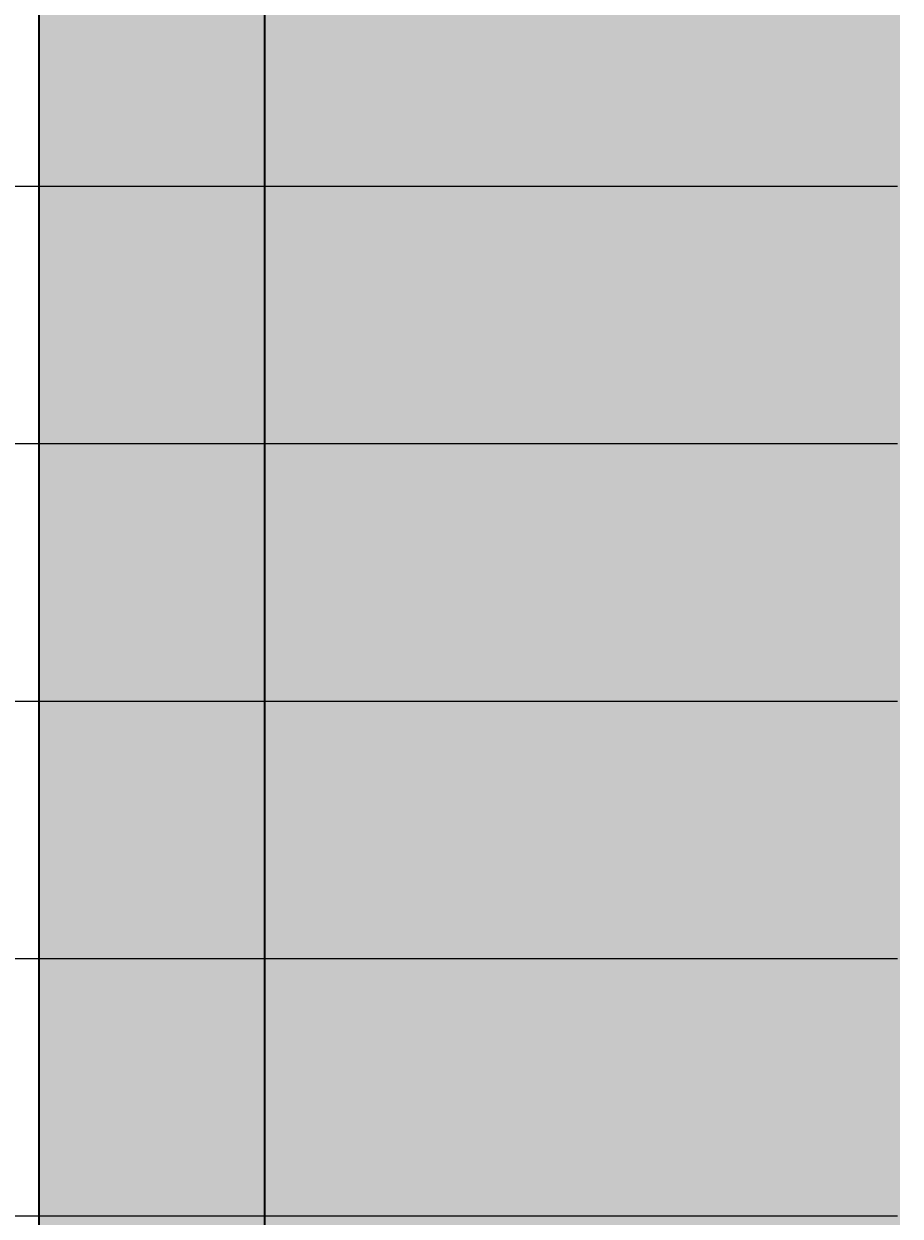
# Model space of a CAD drawing. Units: feet. Extents: x 2695 to 2912, y 795 to 1139.
# Tile 41 of 83: x 2710 to 2731, y 993 to 1020. Entities that reach past the tile are written whole.
import ezdxf

# ---------------------------------------------------------------- set-up
doc = ezdxf.new("R2010")
doc.units = ezdxf.units.FT
for name, color, linetype, lineweight in [('A-ANNO-DIMS', 2, 'Continuous', 18), ('A-ELEV', 7, 'Continuous', 35), ('A-ELEV-PATT', 252, 'Continuous', 13)]:
    doc.layers.add(name, color=color, linetype=linetype, lineweight=lineweight)
doc.styles.get("Standard").update_dxf_attribs({"font": 'arial.ttf'})
doc.dimstyles.get("Standard").update_dxf_attribs({"dimtxt": 0.18, "dimasz": 0.18, "dimexe": 0.18, "dimexo": 0.0625, "dimgap": 0.09, "dimtad": 0, "dimtih": 1, "dimtoh": 1, "dimdec": 1, "dimzin": 0, "dimdsep": 46, "dimlunit": 3, "dimtxsty": 'Standard', "dimcen": 0.09, "dimadec": 0, "dimazin": 0, "dimtfac": 1, "dimtdec": 1, "dimtofl": 0, "dimtmove": 0, "dimatfit": 3, "dimfxl": 1, "dimtolj": 1, "dimtzin": 0, "dimarcsym": 0})

# ---------------------------------------------------------------- blocks, each defined once
blk = doc.blocks.new('*D12')
at = {"layer": 'A-ANNO-DIMS', "color": 0, "lineweight": -2, "transparency": 16777216}
for p, q in [((2710.574, 1122.931), (2694.681, 1122.931)), ((2694.861, 1122.751), (2694.861, 967.113)), ((2694.861, 811.111), (2694.861, 966.749)), ((2710.574, 810.931), (2694.681, 810.931))]:
    blk.add_line(p, q, dxfattribs=at)
at = {"layer": 'A-ANNO-DIMS', "color": 0, "transparency": 16777216}
for points in [[(2694.831, 1122.751), (2694.891, 1122.751), (2694.861, 1122.931)], [(2694.831, 811.111), (2694.891, 811.111), (2694.861, 810.931)]]:
    blk.add_solid(points, dxfattribs=at)
at = {"layer": 'Defpoints', "color": 0, "transparency": 16777216}
for p in [(2694.861, 1122.931), (2710.636, 1122.931), (2710.636, 810.931)]:
    blk.add_point(p, dxfattribs=at)
at = {"layer": 'A-ANNO-DIMS', "color": 0, "transparency": 16777216, "insert": (2694.861, 966.931), "char_height": 0.18, "attachment_point": 5}
blk.add_mtext('\\A1;312', dxfattribs=at)
blk = doc.blocks.new('*D36')
at = {"layer": 'A-ANNO-DIMS', "color": 0, "lineweight": -2, "transparency": 16777216}
for p, q in [((2730.646, 992.518), (2694.681, 992.518)), ((2694.861, 992.338), (2694.861, 989.7)), ((2694.861, 986.698), (2694.861, 989.336)), ((2730.646, 986.518), (2694.681, 986.518))]:
    blk.add_line(p, q, dxfattribs=at)
at = {"layer": 'A-ANNO-DIMS', "color": 0, "transparency": 16777216}
for points in [[(2694.831, 992.338), (2694.891, 992.338), (2694.861, 992.518)], [(2694.831, 986.698), (2694.891, 986.698), (2694.861, 986.518)]]:
    blk.add_solid(points, dxfattribs=at)
at = {"layer": 'Defpoints', "color": 0, "transparency": 16777216}
for p in [(2694.861, 992.518), (2730.708, 992.518), (2730.708, 986.518)]:
    blk.add_point(p, dxfattribs=at)
at = {"layer": 'A-ANNO-DIMS', "color": 0, "transparency": 16777216, "insert": (2694.861, 989.518), "char_height": 0.18, "attachment_point": 5}
blk.add_mtext('\\A1;6', dxfattribs=at)
blk = doc.blocks.new('*D37')
at = {"layer": 'A-ANNO-DIMS', "color": 0, "lineweight": -2, "transparency": 16777216}
for p, q in [((2730.646, 998.518), (2694.681, 998.518)), ((2694.861, 998.338), (2694.861, 995.7)), ((2694.861, 992.698), (2694.861, 995.336)), ((2730.646, 992.518), (2694.681, 992.518))]:
    blk.add_line(p, q, dxfattribs=at)
at = {"layer": 'A-ANNO-DIMS', "color": 0, "transparency": 16777216}
for points in [[(2694.831, 998.338), (2694.891, 998.338), (2694.861, 998.518)], [(2694.831, 992.698), (2694.891, 992.698), (2694.861, 992.518)]]:
    blk.add_solid(points, dxfattribs=at)
at = {"layer": 'Defpoints', "color": 0, "transparency": 16777216}
for p in [(2694.861, 998.518), (2730.708, 998.518), (2730.708, 992.518)]:
    blk.add_point(p, dxfattribs=at)
at = {"layer": 'A-ANNO-DIMS', "color": 0, "transparency": 16777216, "insert": (2694.861, 995.518), "char_height": 0.18, "attachment_point": 5}
blk.add_mtext('\\A1;6', dxfattribs=at)
blk = doc.blocks.new('*D38')
at = {"layer": 'A-ANNO-DIMS', "color": 0, "lineweight": -2, "transparency": 16777216}
for p, q in [((2730.646, 1004.518), (2694.681, 1004.518)), ((2694.861, 1004.338), (2694.861, 1001.7)), ((2694.861, 998.698), (2694.861, 1001.336)), ((2730.646, 998.518), (2694.681, 998.518))]:
    blk.add_line(p, q, dxfattribs=at)
at = {"layer": 'A-ANNO-DIMS', "color": 0, "transparency": 16777216}
for points in [[(2694.831, 1004.338), (2694.891, 1004.338), (2694.861, 1004.518)], [(2694.831, 998.698), (2694.891, 998.698), (2694.861, 998.518)]]:
    blk.add_solid(points, dxfattribs=at)
at = {"layer": 'Defpoints', "color": 0, "transparency": 16777216}
for p in [(2694.861, 1004.518), (2730.708, 1004.518), (2730.708, 998.518)]:
    blk.add_point(p, dxfattribs=at)
at = {"layer": 'A-ANNO-DIMS', "color": 0, "transparency": 16777216, "insert": (2694.861, 1001.518), "char_height": 0.18, "attachment_point": 5}
blk.add_mtext('\\A1;6', dxfattribs=at)
blk = doc.blocks.new('*D39')
at = {"layer": 'A-ANNO-DIMS', "color": 0, "lineweight": -2, "transparency": 16777216}
for p, q in [((2730.646, 1010.518), (2694.681, 1010.518)), ((2694.861, 1010.338), (2694.861, 1007.7)), ((2694.861, 1004.698), (2694.861, 1007.336)), ((2730.646, 1004.518), (2694.681, 1004.518))]:
    blk.add_line(p, q, dxfattribs=at)
at = {"layer": 'A-ANNO-DIMS', "color": 0, "transparency": 16777216}
for points in [[(2694.831, 1010.338), (2694.891, 1010.338), (2694.861, 1010.518)], [(2694.831, 1004.698), (2694.891, 1004.698), (2694.861, 1004.518)]]:
    blk.add_solid(points, dxfattribs=at)
at = {"layer": 'Defpoints', "color": 0, "transparency": 16777216}
for p in [(2694.861, 1010.518), (2730.708, 1010.518), (2730.708, 1004.518)]:
    blk.add_point(p, dxfattribs=at)
at = {"layer": 'A-ANNO-DIMS', "color": 0, "transparency": 16777216, "insert": (2694.861, 1007.518), "char_height": 0.18, "attachment_point": 5}
blk.add_mtext('\\A1;6', dxfattribs=at)
blk = doc.blocks.new('*D40')
at = {"layer": 'A-ANNO-DIMS', "color": 0, "lineweight": -2, "transparency": 16777216}
for p, q in [((2730.646, 1016.518), (2694.681, 1016.518)), ((2694.861, 1016.338), (2694.861, 1013.7)), ((2694.861, 1010.698), (2694.861, 1013.336)), ((2730.646, 1010.518), (2694.681, 1010.518))]:
    blk.add_line(p, q, dxfattribs=at)
at = {"layer": 'A-ANNO-DIMS', "color": 0, "transparency": 16777216}
for points in [[(2694.831, 1016.338), (2694.891, 1016.338), (2694.861, 1016.518)], [(2694.831, 1010.698), (2694.891, 1010.698), (2694.861, 1010.518)]]:
    blk.add_solid(points, dxfattribs=at)
at = {"layer": 'Defpoints', "color": 0, "transparency": 16777216}
for p in [(2694.861, 1016.518), (2730.708, 1016.518), (2730.708, 1010.518)]:
    blk.add_point(p, dxfattribs=at)
at = {"layer": 'A-ANNO-DIMS', "color": 0, "transparency": 16777216, "insert": (2694.861, 1013.518), "char_height": 0.18, "attachment_point": 5}
blk.add_mtext('\\A1;6', dxfattribs=at)
blk = doc.blocks.new('*D41')
at = {"layer": 'A-ANNO-DIMS', "color": 0, "lineweight": -2, "transparency": 16777216}
for p, q in [((2730.646, 1022.518), (2694.681, 1022.518)), ((2694.861, 1022.338), (2694.861, 1019.7)), ((2694.861, 1016.698), (2694.861, 1019.336)), ((2730.646, 1016.518), (2694.681, 1016.518))]:
    blk.add_line(p, q, dxfattribs=at)
at = {"layer": 'A-ANNO-DIMS', "color": 0, "transparency": 16777216}
for points in [[(2694.831, 1022.338), (2694.891, 1022.338), (2694.861, 1022.518)], [(2694.831, 1016.698), (2694.891, 1016.698), (2694.861, 1016.518)]]:
    blk.add_solid(points, dxfattribs=at)
at = {"layer": 'Defpoints', "color": 0, "transparency": 16777216}
for p in [(2694.861, 1022.518), (2730.708, 1022.518), (2730.708, 1016.518)]:
    blk.add_point(p, dxfattribs=at)
at = {"layer": 'A-ANNO-DIMS', "color": 0, "transparency": 16777216, "insert": (2694.861, 1019.518), "char_height": 0.18, "attachment_point": 5}
blk.add_mtext('\\A1;6', dxfattribs=at)

msp = doc.modelspace()

# ---------------------------------------------------------------- hatches: boundary and pattern name
at = {"layer": 'A-ELEV-PATT'}
h = msp.add_hatch(color=256, dxfattribs=at)
h.set_gradient(color1=(255, 255, 255), tint=1)
h.paths.add_polyline_path([(2770.6361, 1122.9306), (2710.6361, 1122.9306), (2710.6361, 1118.4096), (2770.6361, 1118.4096)])
h.paths.add_polyline_path([(2890.6361, 1107.8588), (2770.6361, 1107.8588), (2770.6361, 1103.3378), (2890.6361, 1103.3378)])
h.paths.add_polyline_path([(2890.6361, 1062.9306), (2710.6361, 1062.9306), (2710.6361, 1056.9306), (2710.6361, 936.9306), (2710.6361, 924.3105), (2716.5358, 924.3105), (2890.6361, 924.3105), (2890.6361, 936.9306), (2715.8852, 936.9306), (2715.8852, 1050.3105), (2890.6361, 1050.3105)])
h.paths.add_polyline_path([(2716.5358, 924.3105), (2710.6361, 924.3105), (2710.6361, 810.9306), (2716.5358, 810.9306)])
h = msp.add_hatch(color=256, dxfattribs=at)
h.set_gradient(color1=(147, 149, 152), color2=(147, 149, 152), tint=1)
h.paths.add_polyline_path([(2770.6361, 1118.4096), (2710.6361, 1118.4096), (2710.6361, 1062.9306), (2770.6361, 1062.9306)])
h.paths.add_polyline_path([(2890.6361, 1103.3378), (2770.6361, 1103.3378), (2770.6361, 1062.9306), (2890.6361, 1062.9306)])
h.paths.add_polyline_path([(2730.7081, 1048.1052), (2755.1125, 1048.1052), (2755.1125, 936.9306), (2770.6361, 936.9306), (2770.6361, 1050.3105), (2715.8852, 1050.3105), (2715.8852, 936.9306), (2730.7081, 936.9306)])
h.paths.add_polyline_path([(2890.6361, 1050.3105), (2770.6361, 1050.3105), (2770.6361, 971.9673), (2778.0341, 971.9673), (2778.0341, 1020.8235), (2843.575, 1020.8235), (2843.575, 971.9673), (2890.6361, 971.9673)])
h.paths.add_polyline_path([(2888.1882, 970.7156), (2843.575, 970.7156), (2843.575, 964.8267), (2888.1882, 964.8267)])
h.paths.add_polyline_path([(2888.1882, 964.1328), (2843.575, 964.1328), (2843.575, 956.614), (2888.1882, 956.614)])
h.paths.add_polyline_path([(2888.1882, 955.9202), (2843.575, 955.9202), (2843.575, 949.2892), (2888.1882, 949.2892)])
h.paths.add_polyline_path([(2888.1882, 948.5954), (2843.575, 948.5954), (2843.575, 941.3507), (2888.1882, 941.3507)])
h.paths.add_polyline_path([(2888.1882, 940.6569), (2843.575, 940.6569), (2843.575, 936.9306), (2888.1882, 936.9306)])
h.paths.add_polyline_path([(2890.6361, 970.7156), (2888.9368, 970.7156), (2888.9368, 964.8267), (2890.6361, 964.8267)])
h.paths.add_polyline_path([(2890.6361, 964.1328), (2888.9368, 964.1328), (2888.9368, 956.614), (2890.6361, 956.614)])
h.paths.add_polyline_path([(2890.6361, 955.9202), (2888.9368, 955.9202), (2888.9368, 949.2892), (2890.6361, 949.2892)])
h.paths.add_polyline_path([(2890.6361, 940.6569), (2888.9368, 940.6569), (2888.9368, 936.9306), (2890.6361, 936.9306)])
h.paths.add_polyline_path([(2890.6361, 948.5954), (2888.9368, 948.5954), (2888.9368, 941.3507), (2890.6361, 941.3507)])
h.paths.add_polyline_path([(2772.5216, 970.7156), (2770.6361, 970.7156), (2770.6361, 964.8267), (2772.5216, 964.8267)])
h.paths.add_polyline_path([(2772.5216, 964.1328), (2770.6361, 964.1328), (2770.6361, 956.614), (2772.5216, 956.614)])
h.paths.add_polyline_path([(2772.5216, 955.9202), (2770.6361, 955.9202), (2770.6361, 949.2892), (2772.5216, 949.2892)])
h.paths.add_polyline_path([(2772.5216, 948.5954), (2770.6361, 948.5954), (2770.6361, 941.3507), (2772.5216, 941.3507)])
h.paths.add_polyline_path([(2772.5216, 940.6569), (2770.6361, 940.6569), (2770.6361, 936.9306), (2772.5216, 936.9306)])
h.paths.add_polyline_path([(2778.0341, 940.6569), (2773.2702, 940.6569), (2773.2702, 936.9306), (2778.0341, 936.9306)])
h.paths.add_polyline_path([(2778.0341, 970.7156), (2773.2702, 970.7156), (2773.2702, 964.8267), (2778.0341, 964.8267)])
h.paths.add_polyline_path([(2778.0341, 964.1328), (2773.2702, 964.1328), (2773.2702, 956.614), (2778.0341, 956.614)])
h.paths.add_polyline_path([(2778.0341, 955.9202), (2773.2702, 955.9202), (2773.2702, 949.2892), (2778.0341, 949.2892)])
h.paths.add_polyline_path([(2778.0341, 948.5954), (2773.2702, 948.5954), (2773.2702, 941.3507), (2778.0341, 941.3507)])
h.paths.add_polyline_path([(2810.0407, 940.6569), (2780.0341, 940.6569), (2780.0341, 936.9306), (2810.0407, 936.9306)])
h.paths.add_polyline_path([(2890.6361, 924.3105), (2770.6361, 924.3105), (2770.6361, 810.9306), (2773.5029, 810.9306), (2773.5029, 905.5143), (2805.9398, 905.5143), (2838.3767, 905.5143), (2838.3767, 810.9306), (2890.6361, 810.9306)])

# ---------------------------------------------------------------- linework, layer by layer
at = {"layer": 'A-ELEV'}
for p, q in [((2710.6361, 936.9306), (2710.6361, 1056.9306)), ((2715.8852, 1050.3105), (2715.8852, 936.9306))]:
    msp.add_line(p, q, dxfattribs=at)
msp.add_lwpolyline([(2715.8852, 1050.3105), (2715.8852, 936.9306)], dxfattribs=at)

# ---------------------------------------------------------------- dimensions: what is measured, and where the dimension line sits
at = {"layer": 'A-ANNO-DIMS'}
for base, p1, p2, picture, middle in [((2694.8611, 1122.9306), (2710.6361, 810.9306), (2710.6361, 1122.9306), '*D12', (2694.8611, 966.9306)), ((2694.8611, 1022.5179), (2730.7081, 1016.5179), (2730.7081, 1022.5179), '*D41', (2694.8611, 1019.5179)), ((2694.8611, 1016.5179), (2730.7081, 1010.5179), (2730.7081, 1016.5179), '*D40', (2694.8611, 1013.5179)), ((2694.8611, 1010.5179), (2730.7081, 1004.5179), (2730.7081, 1010.5179), '*D39', (2694.8611, 1007.5179)), ((2694.8611, 1004.5179), (2730.7081, 998.5179), (2730.7081, 1004.5179), '*D38', (2694.8611, 1001.5179)), ((2694.8611, 998.5179), (2730.7081, 992.5179), (2730.7081, 998.5179), '*D37', (2694.8611, 995.5179)), ((2694.8611, 992.5179), (2730.7081, 986.5179), (2730.7081, 992.5179), '*D36', (2694.8611, 989.5179))]:
    dim = msp.add_linear_dim(base=base, p1=p1, p2=p2, angle=90, dimstyle='Standard', override={"dimdec": 0, "dimlfac": 1, "dimrnd": 0, "dimzin": 0, "dimdsep": 46, "dimlunit": 2}, dxfattribs=at)
    dim.commit()
    dim.dimension.update_dxf_attribs({"geometry": picture, "text_midpoint": middle})

doc.saveas('drawing.dxf')
